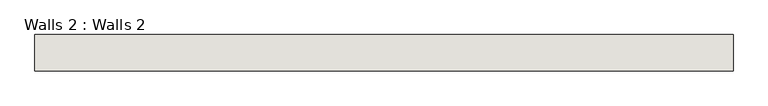
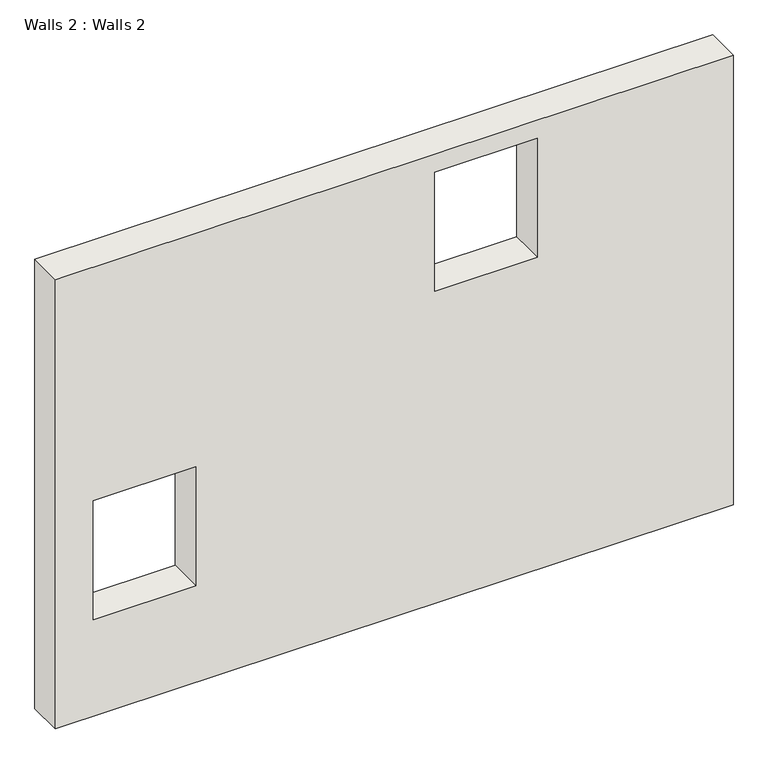
"""IFC4 building model written with IfcOpenShell, lengths in millimetres: wall geometry, Walls 2 : Walls 2."""

from ifc_helpers import new_model, si_unit, frame, origin, place, context, project, spatial, polyline, outline, extrude, source, transform, mapped, element, save


def walls_2_walls_2_fb44fb4a(model_context):
    return source(origin(), model_context, "Body", "SweptSolid", [
        extrude(outline(polyline([(0.0, -15456.4019361), (0.0, -8498.4019361), (4876.8, -8498.4019361), (4876.8, -15456.4019361), (0.0, -15456.4019361)]), holes=[polyline([(2340.5881187, -14014.9519361), (1051.5381187, -14014.9519361), (1051.5381187, -15069.0519361), (2340.5881187, -15069.0519361), (2340.5881187, -14014.9519361)]), polyline([(4679.4605054, -10509.7519361), (3390.4105054, -10509.7519361), (3390.4105054, -11563.8519361), (4679.4605054, -11563.8519361), (4679.4605054, -10509.7519361)])]), frame((0.0, -6969.7875967, 0.0), z_axis=(0.0, 1.0, 0.0), x_axis=(0.0, 0.0, 1.0)), (0.0, 0.0, 1.0), 363.9313053),
    ])


if __name__ == "__main__":
    model = new_model("IFC4")
    model_context = context("Model", 3, world=origin())
    ifc_project = project(units=[si_unit("LENGTHUNIT", "METRE", prefix="MILLI")], contexts=[model_context])
    site = spatial("IfcSite", under=ifc_project)
    building = spatial("IfcBuilding", under=site)
    placement = place(None, origin())
    walls_2_walls_2_shape = walls_2_walls_2_fb44fb4a(model_context)
    element("IfcWall", 1, ObjectType="Walls 2 : Walls 2", at=placement, inside=building, context=model_context, shape_type="MappedRepresentation", body=[
        mapped(walls_2_walls_2_shape, transform((0.0, 0.0, 0.0), x_axis=(1.0, 0.0, 0.0), y_axis=(0.0, 1.0, 0.0), z_axis=(0.0, 0.0, 1.0))),
    ])
    save(model, "model.ifc")

# Revit data of these elements
# Element 1 (IfcWall, "Walls 2 : Walls 2")
#   Materials on its faces: "Default Wall"
# Materials
#   "Default Wall": colour RGB 80 80 80, transparency 0
